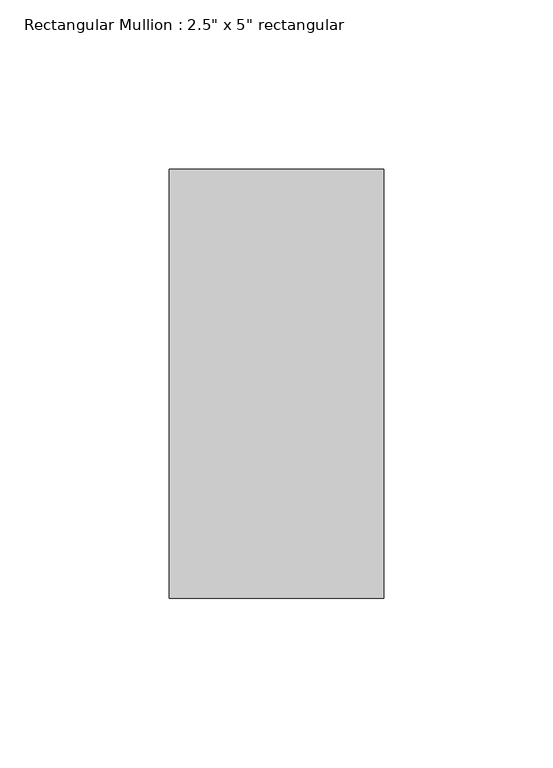
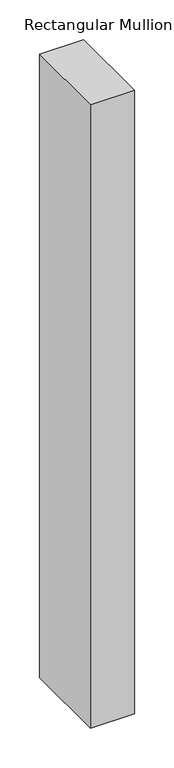
"""IFC4 building model written with IfcOpenShell, lengths in millimetres: member geometry."""

from ifc_helpers import new_model, si_unit, frame, origin, place, context, project, spatial, polyline, outline, extrude, source, transform, mapped, element, save


def member_04c9b82a(model_context):
    return source(origin(), model_context, "Body", "SweptSolid", [
        extrude(outline(polyline([(0.0, 63.5), (0.0, -63.5), (-63.5, -63.5), (-63.5, 63.5), (0.0, 63.5)])), frame((0.0, 0.0, -952.7117553), z_axis=(0.0, 0.0, 1.0), x_axis=(1.0, 0.0, 0.0)), (0.0, 0.0, 1.0), 952.7117553),
    ])


if __name__ == "__main__":
    model = new_model("IFC4")
    model_context = context("Model", 3, world=origin())
    ifc_project = project(units=[si_unit("LENGTHUNIT", "METRE", prefix="MILLI")], contexts=[model_context])
    site = spatial("IfcSite", under=ifc_project)
    building = spatial("IfcBuilding", under=site)
    placement = place(None, origin())
    member_shape = member_04c9b82a(model_context)
    element("IfcMember", 1, ObjectType="Rectangular Mullion : 2.5\" x 5\" rectangular", at=placement, inside=building, context=model_context, shape_type="MappedRepresentation", body=[
        mapped(member_shape, transform((0.0, 0.0, 0.0), x_axis=(1.0, 0.0, 0.0), y_axis=(0.0, 1.0, 0.0), z_axis=(0.0, 0.0, 1.0))),
    ])
    save(model, "model.ifc")

# Revit data of these elements
# Type "Rectangular Mullion : 2.5\" x 5\" rectangular"
#   built-in parameter 1007304 = 0.416667 (stored number, unit not read)
#   built-in parameter 1007301 = 0.104167 (stored number, unit not read)
#   built-in parameter 1007300 = 0.104167 (stored number, unit not read)
# Element 1 (IfcMember, "Rectangular Mullion : 2.5\" x 5\" rectangular")
#   Materials on its faces: "Aluminum"
# Materials
#   "Aluminum": class "Metal", colour RGB 247 247 247, transparency 0, Description = "Aluminum 6061", Cost = 0
